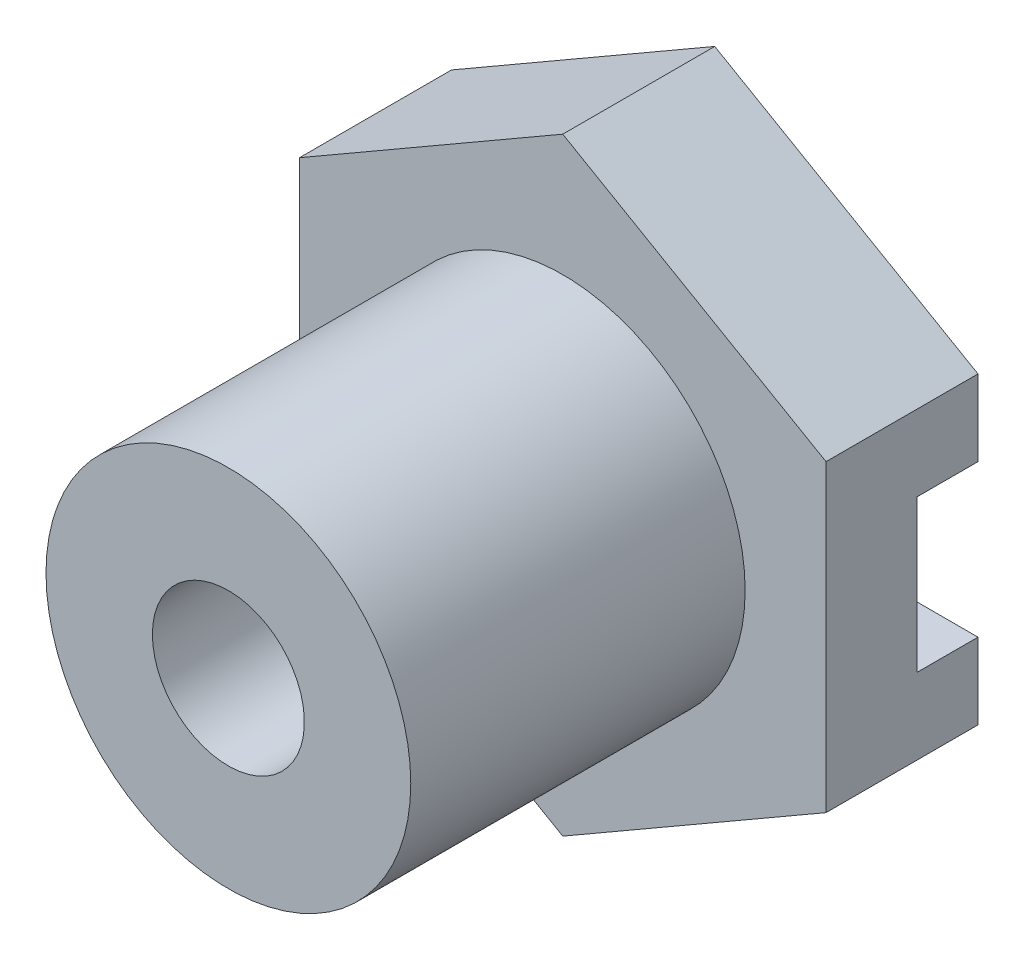
ISO-10303-21;
HEADER;
FILE_DESCRIPTION(('STEP AP214'),'2;1');
FILE_NAME('part.step','',(''),(''),'','','');
FILE_SCHEMA(('AUTOMOTIVE_DESIGN { 1 0 10303 214 1 1 1 1 }'));
ENDSEC;
DATA;
#1=APPLICATION_CONTEXT('core data for automotive mechanical design processes');
#2=APPLICATION_PROTOCOL_DEFINITION('international standard','automotive_design',2000,#1);
#3=PRODUCT_CONTEXT('',#1,'mechanical');
#4=PRODUCT('Part','Part','',(#3));
#5=PRODUCT_RELATED_PRODUCT_CATEGORY('part','',(#4));
#6=PRODUCT_DEFINITION_FORMATION('','',#4);
#7=PRODUCT_DEFINITION_CONTEXT('part definition',#1,'design');
#8=PRODUCT_DEFINITION('design','',#6,#7);
#9=PRODUCT_DEFINITION_SHAPE('','',#8);
#10=(LENGTH_UNIT() NAMED_UNIT(*) SI_UNIT(.MILLI.,.METRE.));
#11=(NAMED_UNIT(*) PLANE_ANGLE_UNIT() SI_UNIT($,.RADIAN.));
#12=(NAMED_UNIT(*) SI_UNIT($,.STERADIAN.) SOLID_ANGLE_UNIT());
#13=UNCERTAINTY_MEASURE_WITH_UNIT(LENGTH_MEASURE(1.E-05),#10,'distance_accuracy_value','');
#14=(GEOMETRIC_REPRESENTATION_CONTEXT(3) GLOBAL_UNCERTAINTY_ASSIGNED_CONTEXT((#13)) GLOBAL_UNIT_ASSIGNED_CONTEXT((#10,
#11,#12)) REPRESENTATION_CONTEXT('',''));
#15=CARTESIAN_POINT('',(0.,0.,0.));
#16=DIRECTION('',(0.,0.,1.));
#17=DIRECTION('',(1.,0.,0.));
#18=AXIS2_PLACEMENT_3D('',#15,#16,#17);
#19=CARTESIAN_POINT('',(0.,0.,2.));
#20=DIRECTION('',(0.,0.,-1.));
#21=DIRECTION('',(-1.,0.,0.));
#22=AXIS2_PLACEMENT_3D('',#19,#20,#21);
#23=PLANE('',#22);
#24=CARTESIAN_POINT('',(0.,0.,2.));
#25=DIRECTION('',(0.,0.,-1.));
#26=DIRECTION('',(-1.,0.,0.));
#27=AXIS2_PLACEMENT_3D('',#24,#25,#26);
#28=CIRCLE('',#27,2.5);
#29=CARTESIAN_POINT('',(0.,2.5,2.));
#30=VERTEX_POINT('',#29);
#31=CARTESIAN_POINT('',(0.,-2.5,2.));
#32=VERTEX_POINT('',#31);
#33=EDGE_CURVE('E53',#30,#32,#28,.T.);
#34=ORIENTED_EDGE('',*,*,#33,.F.);
#35=DIRECTION('',(1.,0.,0.));
#36=VECTOR('',#35,1.);
#37=CARTESIAN_POINT('',(8.66025403784439,2.5,2.));
#38=LINE('',#37,#36);
#39=CARTESIAN_POINT('',(8.66025403784435,2.5,2.));
#40=VERTEX_POINT('',#39);
#41=EDGE_CURVE('E63',#30,#40,#38,.T.);
#42=ORIENTED_EDGE('',*,*,#41,.T.);
#43=DIRECTION('',(0.,-1.,0.));
#44=VECTOR('',#43,1.);
#45=CARTESIAN_POINT('',(8.66025403784439,2.5,2.));
#46=LINE('',#45,#44);
#47=CARTESIAN_POINT('',(8.66025403784439,-2.5,2.));
#48=VERTEX_POINT('',#47);
#49=EDGE_CURVE('E142',#40,#48,#46,.T.);
#50=ORIENTED_EDGE('',*,*,#49,.T.);
#51=DIRECTION('',(-1.,0.,0.));
#52=VECTOR('',#51,1.);
#53=CARTESIAN_POINT('',(8.66025403784439,-2.5,2.));
#54=LINE('',#53,#52);
#55=EDGE_CURVE('E126',#48,#32,#54,.T.);
#56=ORIENTED_EDGE('',*,*,#55,.T.);
#57=EDGE_LOOP('',(#34,#42,#50,#56));
#58=FACE_BOUND('',#57,.T.);
#59=ADVANCED_FACE('F39',(#58),#23,.T.);
#60=CARTESIAN_POINT('',(0.,0.,0.));
#61=DIRECTION('',(0.,0.,1.));
#62=DIRECTION('',(1.,0.,0.));
#63=AXIS2_PLACEMENT_3D('',#60,#61,#62);
#64=PLANE('',#63);
#65=DIRECTION('',(1.,0.,0.));
#66=VECTOR('',#65,1.);
#67=CARTESIAN_POINT('',(8.66025403784439,2.5,0.));
#68=LINE('',#67,#66);
#69=CARTESIAN_POINT('',(-8.66025403784439,2.5,0.));
#70=VERTEX_POINT('',#69);
#71=CARTESIAN_POINT('',(8.66025403784439,2.5,0.));
#72=VERTEX_POINT('',#71);
#73=EDGE_CURVE('E149',#70,#72,#68,.T.);
#74=ORIENTED_EDGE('',*,*,#73,.F.);
#75=DIRECTION('',(0.,-1.,0.));
#76=VECTOR('',#75,1.);
#77=CARTESIAN_POINT('',(-8.66025403784439,4.99999999999998,0.));
#78=LINE('',#77,#76);
#79=CARTESIAN_POINT('',(-8.66025403784439,4.99999999999998,0.));
#80=VERTEX_POINT('',#79);
#81=EDGE_CURVE('E184',#80,#70,#78,.T.);
#82=ORIENTED_EDGE('',*,*,#81,.F.);
#83=DIRECTION('',(-0.866025403784438,-0.500000000000001,0.));
#84=VECTOR('',#83,1.);
#85=CARTESIAN_POINT('',(0.,9.99999999999999,0.));
#86=LINE('',#85,#84);
#87=CARTESIAN_POINT('',(0.,9.99999999999999,0.));
#88=VERTEX_POINT('',#87);
#89=EDGE_CURVE('E182',#88,#80,#86,.T.);
#90=ORIENTED_EDGE('',*,*,#89,.F.);
#91=DIRECTION('',(-0.866025403784442,0.499999999999995,0.));
#92=VECTOR('',#91,1.);
#93=CARTESIAN_POINT('',(8.66025403784432,5.0000000000001,0.));
#94=LINE('',#93,#92);
#95=CARTESIAN_POINT('',(8.66025403784432,5.0000000000001,0.));
#96=VERTEX_POINT('',#95);
#97=EDGE_CURVE('E165',#96,#88,#94,.T.);
#98=ORIENTED_EDGE('',*,*,#97,.F.);
#99=DIRECTION('',(0.,1.,0.));
#100=VECTOR('',#99,1.);
#101=CARTESIAN_POINT('',(8.66025403784443,-4.99999999999992,0.));
#102=LINE('',#101,#100);
#103=EDGE_CURVE('E191',#72,#96,#102,.T.);
#104=ORIENTED_EDGE('',*,*,#103,.F.);
#105=EDGE_LOOP('',(#74,#82,#90,#98,#104));
#106=FACE_BOUND('',#105,.T.);
#107=ADVANCED_FACE('F222',(#106),#64,.F.);
#108=DIRECTION('',(-1.,0.,0.));
#109=VECTOR('',#108,1.);
#110=CARTESIAN_POINT('',(8.66025403784439,-2.5,0.));
#111=LINE('',#110,#109);
#112=CARTESIAN_POINT('',(8.66025403784439,-2.5,0.));
#113=VERTEX_POINT('',#112);
#114=CARTESIAN_POINT('',(-8.66025403784439,-2.5,0.));
#115=VERTEX_POINT('',#114);
#116=EDGE_CURVE('E151',#113,#115,#111,.T.);
#117=ORIENTED_EDGE('',*,*,#116,.F.);
#118=CARTESIAN_POINT('',(8.66025403784443,-4.99999999999992,0.));
#119=VERTEX_POINT('',#118);
#120=EDGE_CURVE('E169',#119,#113,#102,.T.);
#121=ORIENTED_EDGE('',*,*,#120,.F.);
#122=DIRECTION('',(0.866025403784435,0.500000000000007,0.));
#123=VECTOR('',#122,1.);
#124=CARTESIAN_POINT('',(0.,-9.99999999999999,0.));
#125=LINE('',#124,#123);
#126=CARTESIAN_POINT('',(0.,-9.99999999999999,0.));
#127=VERTEX_POINT('',#126);
#128=EDGE_CURVE('E189',#127,#119,#125,.T.);
#129=ORIENTED_EDGE('',*,*,#128,.F.);
#130=DIRECTION('',(0.866025403784442,-0.499999999999995,0.));
#131=VECTOR('',#130,1.);
#132=CARTESIAN_POINT('',(-8.66025403784436,-5.00000000000004,0.));
#133=LINE('',#132,#131);
#134=CARTESIAN_POINT('',(-8.66025403784436,-5.00000000000004,0.));
#135=VERTEX_POINT('',#134);
#136=EDGE_CURVE('E190',#135,#127,#133,.T.);
#137=ORIENTED_EDGE('',*,*,#136,.F.);
#138=EDGE_CURVE('E181',#115,#135,#78,.T.);
#139=ORIENTED_EDGE('',*,*,#138,.F.);
#140=EDGE_LOOP('',(#117,#121,#129,#137,#139));
#141=FACE_BOUND('',#140,.T.);
#142=ADVANCED_FACE('F232',(#141),#64,.F.);
#143=CARTESIAN_POINT('',(8.66025403784432,5.0000000000001,5.));
#144=DIRECTION('',(-0.499999999999995,-0.866025403784442,0.));
#145=DIRECTION('',(0.866025403784442,-0.499999999999995,0.));
#146=AXIS2_PLACEMENT_3D('',#143,#144,#145);
#147=PLANE('',#146);
#148=ORIENTED_EDGE('',*,*,#97,.T.);
#149=DIRECTION('',(0.,0.,-1.));
#150=VECTOR('',#149,1.);
#151=CARTESIAN_POINT('',(0.,9.99999999999999,5.));
#152=LINE('',#151,#150);
#153=CARTESIAN_POINT('',(0.,9.99999999999999,5.));
#154=VERTEX_POINT('',#153);
#155=EDGE_CURVE('E43',#154,#88,#152,.T.);
#156=ORIENTED_EDGE('',*,*,#155,.F.);
#157=DIRECTION('',(-0.866025403784442,0.499999999999995,0.));
#158=VECTOR('',#157,1.);
#159=CARTESIAN_POINT('',(8.66025403784432,5.0000000000001,5.));
#160=LINE('',#159,#158);
#161=CARTESIAN_POINT('',(8.66025403784432,5.0000000000001,5.));
#162=VERTEX_POINT('',#161);
#163=EDGE_CURVE('E163',#162,#154,#160,.T.);
#164=ORIENTED_EDGE('',*,*,#163,.F.);
#165=DIRECTION('',(0.,0.,-1.));
#166=VECTOR('',#165,1.);
#167=CARTESIAN_POINT('',(8.66025403784432,5.0000000000001,5.));
#168=LINE('',#167,#166);
#169=EDGE_CURVE('E178',#162,#96,#168,.T.);
#170=ORIENTED_EDGE('',*,*,#169,.T.);
#171=EDGE_LOOP('',(#148,#156,#164,#170));
#172=FACE_BOUND('',#171,.T.);
#173=ADVANCED_FACE('F41',(#172),#147,.F.);
#174=CARTESIAN_POINT('',(0.,9.99999999999999,5.));
#175=DIRECTION('',(0.500000000000001,-0.866025403784438,0.));
#176=DIRECTION('',(0.866025403784438,0.500000000000001,0.));
#177=AXIS2_PLACEMENT_3D('',#174,#175,#176);
#178=PLANE('',#177);
#179=ORIENTED_EDGE('',*,*,#89,.T.);
#180=DIRECTION('',(0.,0.,-1.));
#181=VECTOR('',#180,1.);
#182=CARTESIAN_POINT('',(-8.66025403784439,4.99999999999998,5.));
#183=LINE('',#182,#181);
#184=CARTESIAN_POINT('',(-8.66025403784439,4.99999999999998,5.));
#185=VERTEX_POINT('',#184);
#186=EDGE_CURVE('E204',#185,#80,#183,.T.);
#187=ORIENTED_EDGE('',*,*,#186,.F.);
#188=DIRECTION('',(-0.866025403784438,-0.500000000000001,0.));
#189=VECTOR('',#188,1.);
#190=CARTESIAN_POINT('',(0.,9.99999999999999,5.));
#191=LINE('',#190,#189);
#192=EDGE_CURVE('E170',#154,#185,#191,.T.);
#193=ORIENTED_EDGE('',*,*,#192,.F.);
#194=ORIENTED_EDGE('',*,*,#155,.T.);
#195=EDGE_LOOP('',(#179,#187,#193,#194));
#196=FACE_BOUND('',#195,.T.);
#197=ADVANCED_FACE('F213',(#196),#178,.F.);
#198=CARTESIAN_POINT('',(-8.66025403784439,4.99999999999998,5.));
#199=DIRECTION('',(1.,0.,0.));
#200=DIRECTION('',(0.,1.,0.));
#201=AXIS2_PLACEMENT_3D('',#198,#199,#200);
#202=PLANE('',#201);
#203=DIRECTION('',(0.,1.,0.));
#204=VECTOR('',#203,1.);
#205=CARTESIAN_POINT('',(-8.66025403784439,2.5,2.));
#206=LINE('',#205,#204);
#207=CARTESIAN_POINT('',(-8.66025403784439,-2.5,2.));
#208=VERTEX_POINT('',#207);
#209=CARTESIAN_POINT('',(-8.66025403784439,2.5,2.));
#210=VERTEX_POINT('',#209);
#211=EDGE_CURVE('E140',#208,#210,#206,.T.);
#212=ORIENTED_EDGE('',*,*,#211,.F.);
#213=DIRECTION('',(0.,0.,-1.));
#214=VECTOR('',#213,1.);
#215=CARTESIAN_POINT('',(-8.66025403784439,-2.5,2.));
#216=LINE('',#215,#214);
#217=EDGE_CURVE('E153',#208,#115,#216,.T.);
#218=ORIENTED_EDGE('',*,*,#217,.T.);
#219=ORIENTED_EDGE('',*,*,#138,.T.);
#220=DIRECTION('',(0.,0.,-1.));
#221=VECTOR('',#220,1.);
#222=CARTESIAN_POINT('',(-8.66025403784436,-5.00000000000004,5.));
#223=LINE('',#222,#221);
#224=CARTESIAN_POINT('',(-8.66025403784436,-5.00000000000004,5.));
#225=VERTEX_POINT('',#224);
#226=EDGE_CURVE('E205',#225,#135,#223,.T.);
#227=ORIENTED_EDGE('',*,*,#226,.F.);
#228=DIRECTION('',(0.,-1.,0.));
#229=VECTOR('',#228,1.);
#230=CARTESIAN_POINT('',(-8.66025403784439,4.99999999999998,5.));
#231=LINE('',#230,#229);
#232=EDGE_CURVE('E168',#185,#225,#231,.T.);
#233=ORIENTED_EDGE('',*,*,#232,.F.);
#234=ORIENTED_EDGE('',*,*,#186,.T.);
#235=ORIENTED_EDGE('',*,*,#81,.T.);
#236=DIRECTION('',(0.,0.,-1.));
#237=VECTOR('',#236,1.);
#238=CARTESIAN_POINT('',(-8.66025403784439,2.5,2.));
#239=LINE('',#238,#237);
#240=EDGE_CURVE('E146',#210,#70,#239,.T.);
#241=ORIENTED_EDGE('',*,*,#240,.F.);
#242=EDGE_LOOP('',(#212,#218,#219,#227,#233,#234,#235,#241));
#243=FACE_BOUND('',#242,.T.);
#244=ADVANCED_FACE('F225',(#243),#202,.F.);
#245=CARTESIAN_POINT('',(-8.66025403784436,-5.00000000000004,5.));
#246=DIRECTION('',(0.499999999999995,0.866025403784442,0.));
#247=DIRECTION('',(-0.866025403784442,0.499999999999995,0.));
#248=AXIS2_PLACEMENT_3D('',#245,#246,#247);
#249=PLANE('',#248);
#250=ORIENTED_EDGE('',*,*,#136,.T.);
#251=DIRECTION('',(0.,0.,-1.));
#252=VECTOR('',#251,1.);
#253=CARTESIAN_POINT('',(0.,-9.99999999999999,5.));
#254=LINE('',#253,#252);
#255=CARTESIAN_POINT('',(0.,-9.99999999999999,5.));
#256=VERTEX_POINT('',#255);
#257=EDGE_CURVE('E200',#256,#127,#254,.T.);
#258=ORIENTED_EDGE('',*,*,#257,.F.);
#259=DIRECTION('',(0.866025403784442,-0.499999999999995,0.));
#260=VECTOR('',#259,1.);
#261=CARTESIAN_POINT('',(-8.66025403784436,-5.00000000000004,5.));
#262=LINE('',#261,#260);
#263=EDGE_CURVE('E175',#225,#256,#262,.T.);
#264=ORIENTED_EDGE('',*,*,#263,.F.);
#265=ORIENTED_EDGE('',*,*,#226,.T.);
#266=EDGE_LOOP('',(#250,#258,#264,#265));
#267=FACE_BOUND('',#266,.T.);
#268=ADVANCED_FACE('F239',(#267),#249,.F.);
#269=CARTESIAN_POINT('',(0.,-9.99999999999999,5.));
#270=DIRECTION('',(-0.500000000000007,0.866025403784435,0.));
#271=DIRECTION('',(-0.866025403784435,-0.500000000000007,0.));
#272=AXIS2_PLACEMENT_3D('',#269,#270,#271);
#273=PLANE('',#272);
#274=ORIENTED_EDGE('',*,*,#128,.T.);
#275=DIRECTION('',(0.,0.,-1.));
#276=VECTOR('',#275,1.);
#277=CARTESIAN_POINT('',(8.66025403784443,-4.99999999999992,5.));
#278=LINE('',#277,#276);
#279=CARTESIAN_POINT('',(8.66025403784443,-4.99999999999992,5.));
#280=VERTEX_POINT('',#279);
#281=EDGE_CURVE('E198',#280,#119,#278,.T.);
#282=ORIENTED_EDGE('',*,*,#281,.F.);
#283=DIRECTION('',(0.866025403784435,0.500000000000007,0.));
#284=VECTOR('',#283,1.);
#285=CARTESIAN_POINT('',(0.,-9.99999999999999,5.));
#286=LINE('',#285,#284);
#287=EDGE_CURVE('E174',#256,#280,#286,.T.);
#288=ORIENTED_EDGE('',*,*,#287,.F.);
#289=ORIENTED_EDGE('',*,*,#257,.T.);
#290=EDGE_LOOP('',(#274,#282,#288,#289));
#291=FACE_BOUND('',#290,.T.);
#292=ADVANCED_FACE('F241',(#291),#273,.F.);
#293=CARTESIAN_POINT('',(8.66025403784443,-4.99999999999992,5.));
#294=DIRECTION('',(-1.,0.,0.));
#295=DIRECTION('',(0.,-1.,0.));
#296=AXIS2_PLACEMENT_3D('',#293,#294,#295);
#297=PLANE('',#296);
#298=ORIENTED_EDGE('',*,*,#49,.F.);
#299=DIRECTION('',(0.,0.,-1.));
#300=VECTOR('',#299,1.);
#301=CARTESIAN_POINT('',(8.66025403784439,2.5,2.));
#302=LINE('',#301,#300);
#303=EDGE_CURVE('E132',#40,#72,#302,.T.);
#304=ORIENTED_EDGE('',*,*,#303,.T.);
#305=ORIENTED_EDGE('',*,*,#103,.T.);
#306=ORIENTED_EDGE('',*,*,#169,.F.);
#307=DIRECTION('',(0.,1.,0.));
#308=VECTOR('',#307,1.);
#309=CARTESIAN_POINT('',(8.66025403784443,-4.99999999999992,5.));
#310=LINE('',#309,#308);
#311=EDGE_CURVE('E176',#280,#162,#310,.T.);
#312=ORIENTED_EDGE('',*,*,#311,.F.);
#313=ORIENTED_EDGE('',*,*,#281,.T.);
#314=ORIENTED_EDGE('',*,*,#120,.T.);
#315=DIRECTION('',(0.,0.,-1.));
#316=VECTOR('',#315,1.);
#317=CARTESIAN_POINT('',(8.66025403784439,-2.5,2.));
#318=LINE('',#317,#316);
#319=EDGE_CURVE('E160',#48,#113,#318,.T.);
#320=ORIENTED_EDGE('',*,*,#319,.F.);
#321=EDGE_LOOP('',(#298,#304,#305,#306,#312,#313,#314,#320));
#322=FACE_BOUND('',#321,.T.);
#323=ADVANCED_FACE('F221',(#322),#297,.F.);
#324=CARTESIAN_POINT('',(0.,0.,5.));
#325=DIRECTION('',(0.,0.,1.));
#326=DIRECTION('',(1.,0.,0.));
#327=AXIS2_PLACEMENT_3D('',#324,#325,#326);
#328=PLANE('',#327);
#329=CARTESIAN_POINT('',(0.,0.,5.));
#330=DIRECTION('',(0.,0.,1.));
#331=DIRECTION('',(1.,0.,0.));
#332=AXIS2_PLACEMENT_3D('',#329,#330,#331);
#333=CIRCLE('',#332,6.);
#334=CARTESIAN_POINT('',(6.,0.,5.));
#335=VERTEX_POINT('',#334);
#336=EDGE_CURVE('E11',#335,#335,#333,.T.);
#337=ORIENTED_EDGE('',*,*,#336,.F.);
#338=EDGE_LOOP('',(#337));
#339=FACE_BOUND('',#338,.T.);
#340=ORIENTED_EDGE('',*,*,#163,.T.);
#341=ORIENTED_EDGE('',*,*,#192,.T.);
#342=ORIENTED_EDGE('',*,*,#232,.T.);
#343=ORIENTED_EDGE('',*,*,#263,.T.);
#344=ORIENTED_EDGE('',*,*,#287,.T.);
#345=ORIENTED_EDGE('',*,*,#311,.T.);
#346=EDGE_LOOP('',(#340,#341,#342,#343,#344,#345));
#347=FACE_BOUND('',#346,.T.);
#348=ADVANCED_FACE('F250',(#339,#347),#328,.T.);
#349=CARTESIAN_POINT('',(0.,0.,16.));
#350=DIRECTION('',(0.,0.,-1.));
#351=DIRECTION('',(-1.,0.,0.));
#352=AXIS2_PLACEMENT_3D('',#349,#350,#351);
#353=CYLINDRICAL_SURFACE('',#352,6.);
#354=CARTESIAN_POINT('',(0.,0.,16.));
#355=DIRECTION('',(0.,0.,1.));
#356=DIRECTION('',(1.,0.,0.));
#357=AXIS2_PLACEMENT_3D('',#354,#355,#356);
#358=CIRCLE('',#357,6.);
#359=CARTESIAN_POINT('',(6.,0.,16.));
#360=VERTEX_POINT('',#359);
#361=EDGE_CURVE('E156',#360,#360,#358,.T.);
#362=ORIENTED_EDGE('',*,*,#361,.F.);
#363=EDGE_LOOP('',(#362));
#364=FACE_BOUND('',#363,.T.);
#365=ORIENTED_EDGE('',*,*,#336,.T.);
#366=EDGE_LOOP('',(#365));
#367=FACE_BOUND('',#366,.T.);
#368=ADVANCED_FACE('F247',(#364,#367),#353,.T.);
#369=CARTESIAN_POINT('',(0.,0.,16.));
#370=DIRECTION('',(0.,0.,1.));
#371=DIRECTION('',(1.,0.,0.));
#372=AXIS2_PLACEMENT_3D('',#369,#370,#371);
#373=PLANE('',#372);
#374=CARTESIAN_POINT('',(0.,0.,16.));
#375=DIRECTION('',(0.,0.,-1.));
#376=DIRECTION('',(-1.,0.,0.));
#377=AXIS2_PLACEMENT_3D('',#374,#375,#376);
#378=CIRCLE('',#377,2.5);
#379=CARTESIAN_POINT('',(-2.5,0.,16.));
#380=VERTEX_POINT('',#379);
#381=EDGE_CURVE('E129',#380,#380,#378,.T.);
#382=ORIENTED_EDGE('',*,*,#381,.T.);
#383=EDGE_LOOP('',(#382));
#384=FACE_BOUND('',#383,.T.);
#385=ORIENTED_EDGE('',*,*,#361,.T.);
#386=EDGE_LOOP('',(#385));
#387=FACE_BOUND('',#386,.T.);
#388=ADVANCED_FACE('F258',(#384,#387),#373,.T.);
#389=CARTESIAN_POINT('',(8.66025403784439,-2.5,2.));
#390=DIRECTION('',(0.,-1.,0.));
#391=DIRECTION('',(0.,0.,-1.));
#392=AXIS2_PLACEMENT_3D('',#389,#390,#391);
#393=PLANE('',#392);
#394=ORIENTED_EDGE('',*,*,#116,.T.);
#395=ORIENTED_EDGE('',*,*,#217,.F.);
#396=EDGE_CURVE('E141',#32,#208,#54,.T.);
#397=ORIENTED_EDGE('',*,*,#396,.F.);
#398=ORIENTED_EDGE('',*,*,#55,.F.);
#399=ORIENTED_EDGE('',*,*,#319,.T.);
#400=EDGE_LOOP('',(#394,#395,#397,#398,#399));
#401=FACE_BOUND('',#400,.T.);
#402=ADVANCED_FACE('F230',(#401),#393,.F.);
#403=CARTESIAN_POINT('',(8.66025403784439,2.5,2.));
#404=DIRECTION('',(0.,1.,0.));
#405=DIRECTION('',(0.,0.,1.));
#406=AXIS2_PLACEMENT_3D('',#403,#404,#405);
#407=PLANE('',#406);
#408=ORIENTED_EDGE('',*,*,#73,.T.);
#409=ORIENTED_EDGE('',*,*,#303,.F.);
#410=ORIENTED_EDGE('',*,*,#41,.F.);
#411=EDGE_CURVE('E135',#210,#30,#38,.T.);
#412=ORIENTED_EDGE('',*,*,#411,.F.);
#413=ORIENTED_EDGE('',*,*,#240,.T.);
#414=EDGE_LOOP('',(#408,#409,#410,#412,#413));
#415=FACE_BOUND('',#414,.T.);
#416=ADVANCED_FACE('F133',(#415),#407,.F.);
#417=EDGE_CURVE('E117',#32,#30,#28,.T.);
#418=ORIENTED_EDGE('',*,*,#417,.F.);
#419=ORIENTED_EDGE('',*,*,#396,.T.);
#420=ORIENTED_EDGE('',*,*,#211,.T.);
#421=ORIENTED_EDGE('',*,*,#411,.T.);
#422=EDGE_LOOP('',(#418,#419,#420,#421));
#423=FACE_BOUND('',#422,.T.);
#424=ADVANCED_FACE('F137',(#423),#23,.T.);
#425=CARTESIAN_POINT('',(0.,0.,16.));
#426=DIRECTION('',(0.,0.,-1.));
#427=DIRECTION('',(-1.,0.,0.));
#428=AXIS2_PLACEMENT_3D('',#425,#426,#427);
#429=CYLINDRICAL_SURFACE('',#428,2.5);
#430=ORIENTED_EDGE('',*,*,#381,.F.);
#431=EDGE_LOOP('',(#430));
#432=FACE_BOUND('',#431,.T.);
#433=ORIENTED_EDGE('',*,*,#33,.T.);
#434=ORIENTED_EDGE('',*,*,#417,.T.);
#435=EDGE_LOOP('',(#433,#434));
#436=FACE_BOUND('',#435,.T.);
#437=ADVANCED_FACE('F121',(#432,#436),#429,.F.);
#438=CLOSED_SHELL('',(#59,#107,#142,#173,#197,#244,#268,#292,#323,#348,#368,#388,#402,#416,#424,#437));
#439=MANIFOLD_SOLID_BREP('B2',#438);
#440=ADVANCED_BREP_SHAPE_REPRESENTATION('',(#18,#439),#14);
#441=SHAPE_DEFINITION_REPRESENTATION(#9,#440);
ENDSEC;
END-ISO-10303-21;
